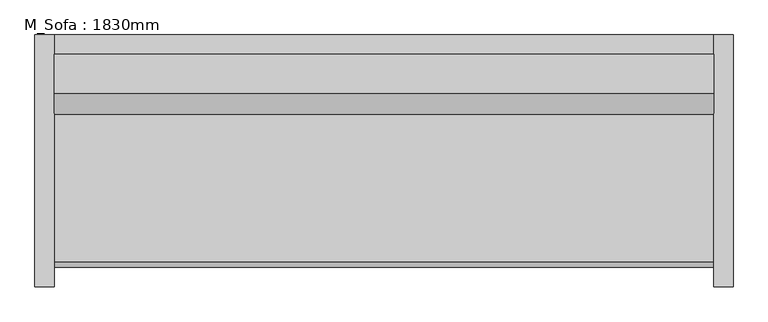
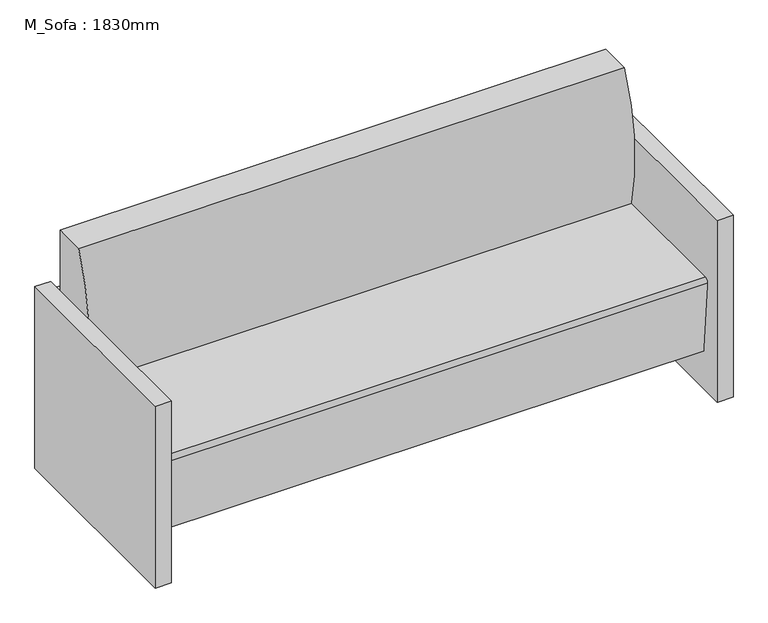
"""IFC4 building model written with IfcOpenShell, lengths in millimetres: furniture geometry, M_Sofa : 1830mm."""

from ifc_helpers import new_model, si_unit, point, frame, frame_2d, origin, origin_with_axes, place, context, project, spatial, polyline, circle_curve, trimmed, segment, composite_curve, outline, extrude, source, transform, mapped, element, save


def m_sofa_1830mm_f9e8a66b(model_context):
    return source(origin(), model_context, "Body", "SweptSolid", [
        extrude(outline(polyline([(-793.8295082, 425.5540984), (-793.8295082, 476.3540984), (934.5704918, 476.3540984), (934.5704918, 425.5540984), (-793.8295082, 425.5540984)])), frame((0.0, 0.0, 457.2), z_axis=(0.0, 0.0, 1.0), x_axis=(1.0, 0.0, 0.0)), (0.0, 0.0, 1.0), 127.0),
        extrude(outline(polyline([(-793.8295082, 425.5540984), (-793.8295082, 476.3540984), (934.5704918, 476.3540984), (934.5704918, 425.5540984), (-793.8295082, 425.5540984)])), frame((0.0, 0.0, 266.7), z_axis=(0.0, 0.0, 1.0), x_axis=(1.0, 0.0, 0.0)), (0.0, 0.0, 1.0), 127.0),
        extrude(outline(polyline([(-793.8295082, 425.5540984), (-793.8295082, 476.3540984), (934.5704918, 476.3540984), (934.5704918, 425.5540984), (-793.8295082, 425.5540984)])), frame((0.0, 0.0, 76.2), z_axis=(0.0, 0.0, 1.0), x_axis=(1.0, 0.0, 0.0)), (0.0, 0.0, 1.0), 127.0),
        extrude(outline(composite_curve([segment(trimmed(circle_curve(frame_2d((926.517198, 542.5300036)), 660.4), [point((286.1764935, 381.0))], [point((323.9540984, 812.8))], False, "CARTESIAN"), True, "CONTINUOUS"), segment(polyline([(323.9540984, 812.8), (425.5540984, 812.8), (425.5540984, 127.9665467), (-111.108343, 127.9665467), (-132.0379563, 367.1931221)]), True, "CONTINUOUS"), segment(trimmed(circle_curve(frame_2d((-119.3862837, 368.3)), 12.7), [point((-132.0379563, 367.1931221))], [point((-119.3862837, 381.0))], False, "CARTESIAN"), True, "CONTINUOUS"), segment(polyline([(-119.3862837, 381.0), (286.1764935, 381.0)]), True, "CONTINUOUS")], self_intersect=False)), frame((-793.8295082, 0.0, 0.0), z_axis=(1.0, 0.0, 0.0), x_axis=(0.0, 1.0, 0.0)), (0.0, 0.0, 1.0), 1728.4),
        extrude(outline(polyline([(-793.8295082, 476.3540984), (-793.8295082, -184.0459016), (-844.6295082, -184.0459016), (-844.6295082, 476.3540984), (-793.8295082, 476.3540984)])), origin_with_axes(), (0.0, 0.0, 1.0), 609.6),
        extrude(outline(polyline([(985.3704918, 476.3540984), (985.3704918, -184.0459016), (934.5704918, -184.0459016), (934.5704918, 476.3540984), (985.3704918, 476.3540984)])), origin_with_axes(), (0.0, 0.0, 1.0), 609.6),
    ])


if __name__ == "__main__":
    model = new_model("IFC4")
    model_context = context("Model", 3, world=origin())
    ifc_project = project(units=[si_unit("LENGTHUNIT", "METRE", prefix="MILLI")], contexts=[model_context])
    site = spatial("IfcSite", under=ifc_project)
    building = spatial("IfcBuilding", under=site)
    placement = place(None, origin())
    m_sofa_1830mm_shape = m_sofa_1830mm_f9e8a66b(model_context)
    element("IfcFurniture", 1, ObjectType="M_Sofa : 1830mm", at=placement, inside=building, context=model_context, shape_type="MappedRepresentation", body=[
        mapped(m_sofa_1830mm_shape, transform((0.0, 0.0, 0.0), x_axis=(1.0, 0.0, 0.0), y_axis=(0.0, 1.0, 0.0), z_axis=(0.0, 0.0, 1.0))),
    ])
    save(model, "model.ifc")

# Revit data of these elements
# Type "M_Sofa : 1830mm"
#   Width = 6' - 0.04724"
#   Seat Material = Linen, Beige
#   Frame Material = Cherry
#   Default Elevation = 0
# Element 1 (IfcFurniture, "M_Sofa : 1830mm")
#   Materials on its faces: "Cherry", "Linen, Beige"
# Materials
#   "Linen, Beige": class "Textile", colour RGB 249 239 230, transparency 0, Description = "Linen, beige", Cost = 0
#   "Cherry": class "Wood", colour RGB 226 177 128, transparency 0, Description = "Prunus Serotina", Cost = 0
